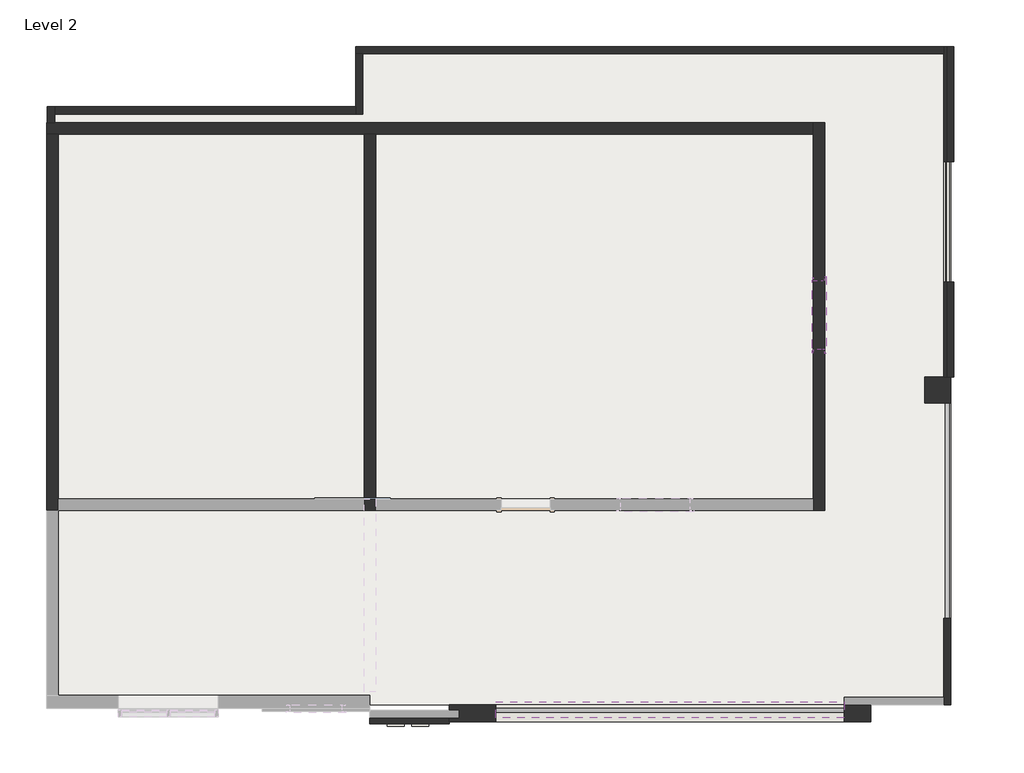
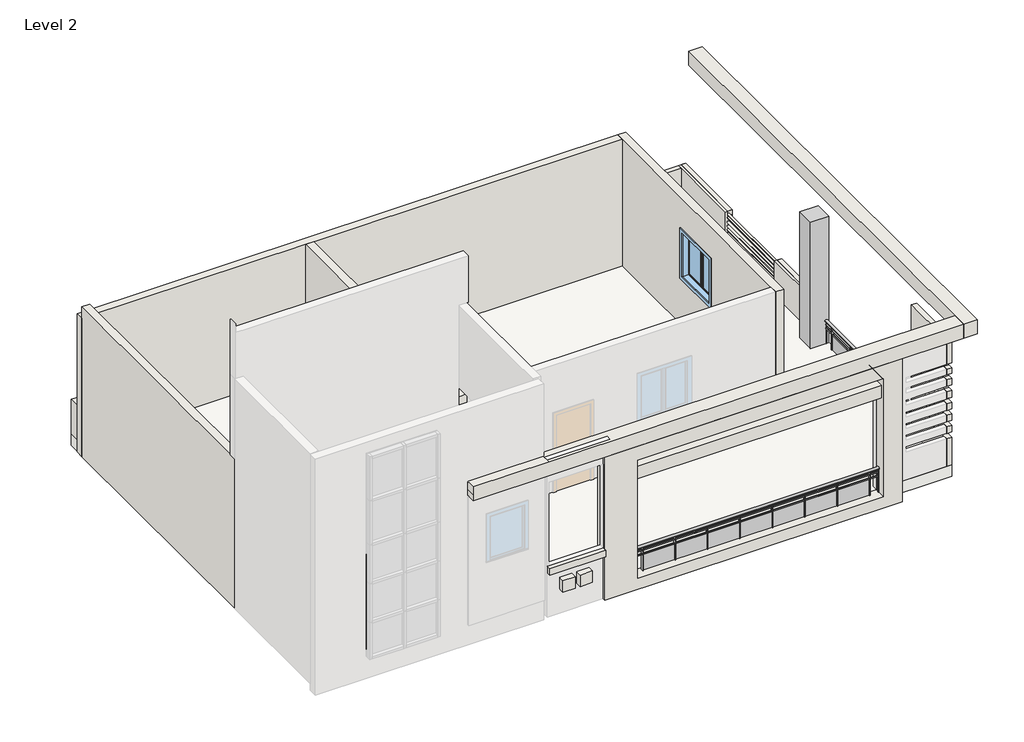
# One storey, part 2 of 2: 16 walls, 2 railings, 1 column, 1 roof, 1 window.
"""IFC4 building model written with IfcOpenShell, lengths in millimetres."""

from ifc_helpers import new_model, si_unit, point, frame, origin, place, context, project, spatial, polyline, ellipse_curve, trimmed, outline, extrude, faceted_brep, transform, mapped, element, save
from ifc_brep_helpers import plane_surface, extruded_surface, advanced_brep
from components import walls_1_walls_1_3d42d239, walls_4_walls_4_4fd3bbeb, walls_5_walls_5_3445876a, walls_6_walls_6_35ebc142, walls_7_walls_7_87e04c6a, walls_8_walls_8_d012f144, window_0862ab64

model = new_model("IFC4")

# Units and contexts
model_context = context("Model", 3, world=origin())
ifc_project = project(units=[si_unit("LENGTHUNIT", "METRE", prefix="MILLI")], contexts=[model_context])

# Site, building, storey
site = spatial("IfcSite", under=ifc_project)
building = spatial("IfcBuilding", under=site)
storey = spatial("IfcBuildingStorey", under=building, Name="Level 2", Elevation=3657.6)

# Column
placement = place(None, origin())
element("IfcColumn", 1, ObjectType="Rectangular Column : 18\" x 18\"", at=placement, inside=storey, context=model_context, shape_type="Brep", body=[
    faceted_brep([(2145.4271302, 2090.1740351, 7315.2), (1688.2271302, 2090.1740351, 7315.2), (1688.2271302, 1632.9740351, 7315.2), (2145.4271302, 1632.9740351, 7315.2), (2145.4271302, 2090.1740351, 3962.4), (2145.4271302, 1632.9740351, 3962.4), (1688.2271302, 1632.9740351, 3962.4), (1688.2271302, 2090.1740351, 3962.4), (2018.4271302, 2090.1740351, 3962.4), (2145.4271302, 2090.1740351, 4876.8)], [[[0, 1, 2, 3]], [[4, 5, 6, 7, 8]], [[1, 0, 9, 4, 8, 7]], [[2, 1, 7, 6]], [[3, 2, 6, 5]], [[0, 3, 5, 4, 9]]]),
])

# Railings
element("IfcRailing", 2, ObjectType="Glass Panel - Bottom Fill", at=placement, inside=storey, context=model_context, shape_type="SolidModel", body=[
    advanced_brep(
    [(-5897.2145744, -3764.5259649, 4605.5359375), (-5897.2145744, -3840.7259649, 4605.5359375), (258.2694807, -3764.5259649, 4605.5359375), (258.2694807, -3840.7259649, 4605.5359375)],
    [
        (0, 1, ellipse_curve(frame((-5897.2145744, -3802.6259649, 4605.5359375), z_axis=(-1.0, 0.0, 0.0), x_axis=(0.0, -1.0, 0.0)), 38.1, 28.575)),
        (1, 0, ellipse_curve(frame((-5897.2145744, -3802.6259649, 4605.5359375), z_axis=(-1.0, 0.0, 0.0), x_axis=(0.0, -1.0, 0.0)), 38.1, 28.575)),
        (2, 3, ellipse_curve(frame((258.2694807, -3802.6259649, 4605.5359375), z_axis=(1.0, 0.0, 0.0), x_axis=(0.0, -1.0, 0.0)), 38.1, 28.575)),
        (3, 2, ellipse_curve(frame((258.2694807, -3802.6259649, 4605.5359375), z_axis=(1.0, 0.0, 0.0), x_axis=(0.0, -1.0, 0.0)), 38.1, 28.575)),
        (0, 2),
        (3, 1),
    ],
    [
        plane_surface(frame((-5897.2145744, -3802.6259649, 4605.5359375), z_axis=(-1.0, 0.0, 0.0), x_axis=(0.0, 1.0, 0.0))),
        plane_surface(frame((258.2694807, -3802.6259649, 4605.5359375), z_axis=(1.0, 0.0, 0.0), x_axis=(0.0, 1.0, 0.0))),
        extruded_surface(trimmed(ellipse_curve(frame((258.2694807, -3802.6259649, 4605.5359375), z_axis=(-1.0, 0.0, 0.0), x_axis=(0.0, -1.0, 0.0)), 38.1, 28.575), [point((258.2694807, -3764.5259649, 4605.5359375))], [point((258.2694807, -3840.7259649, 4605.5359375))], True, "CARTESIAN"), (-6155.4840551, 0.0, 0.0), 6155.4840551),
        extruded_surface(trimmed(ellipse_curve(frame((258.2694807, -3802.6259649, 4605.5359375), z_axis=(-1.0, 0.0, 0.0), x_axis=(0.0, -1.0, 0.0)), 38.1, 28.575), [point((258.2694807, -3840.7259649, 4605.5359375))], [point((258.2694807, -3764.5259649, 4605.5359375))], True, "CARTESIAN"), (-6155.4840551, 0.0, 0.0), 6155.4840551),
    ],
    [
        (0, [[1, 2]]),
        (1, [[3, 4]]),
        (2, [[-1, 5, -4, 6]]),
        (3, [[-2, -6, -3, -5]]),
    ],
),
    extrude(outline(polyline([(-5897.2145744, -3815.3259649), (-5897.2145744, -3789.9259649), (258.2694807, -3789.9259649), (258.2694807, -3815.3259649), (-5897.2145744, -3815.3259649)])), frame((0.0, 0.0, 4491.2359375), z_axis=(0.0, 0.0, 1.0), x_axis=(1.0, 0.0, 0.0)), (0.0, 0.0, 1.0), 25.4),
    extrude(outline(polyline([(-5897.2145744, -3815.3259649), (-5897.2145744, -3789.9259649), (258.2694807, -3789.9259649), (258.2694807, -3815.3259649), (-5897.2145744, -3815.3259649)])), frame((0.0, 0.0, 4389.6359375), z_axis=(0.0, 0.0, 1.0), x_axis=(1.0, 0.0, 0.0)), (0.0, 0.0, 1.0), 25.4),
    extrude(outline(polyline([(18.9774532, -3828.0259649), (18.9774532, -3777.2259649), (31.6774532, -3777.2259649), (31.6774532, -3828.0259649), (18.9774532, -3828.0259649)])), frame((0.0, 0.0, 3691.1359375), z_axis=(0.0, 0.0, 1.0), x_axis=(1.0, 0.0, 0.0)), (0.0, 0.0, 1.0), 885.6788223),
    extrude(outline(polyline([(-787.4725468, -3796.0908079), (25.3274532, -3796.0908079), (25.3274532, -3802.4408079), (-787.4725468, -3802.4408079), (-787.4725468, -3796.0908079)])), frame((0.0, 0.0, 3792.7359375), z_axis=(0.0, 0.0, 1.0), x_axis=(1.0, 0.0, 0.0)), (0.0, 0.0, 1.0), 596.9),
    extrude(outline(polyline([(-793.8225468, -3828.0259649), (-793.8225468, -3777.2259649), (-781.1225468, -3777.2259649), (-781.1225468, -3828.0259649), (-793.8225468, -3828.0259649)])), frame((0.0, 0.0, 3691.1359375), z_axis=(0.0, 0.0, 1.0), x_axis=(1.0, 0.0, 0.0)), (0.0, 0.0, 1.0), 885.6788223),
    extrude(outline(polyline([(-1600.2725468, -3796.0908079), (-787.4725468, -3796.0908079), (-787.4725468, -3802.4408079), (-1600.2725468, -3802.4408079), (-1600.2725468, -3796.0908079)])), frame((0.0, 0.0, 3792.7359375), z_axis=(0.0, 0.0, 1.0), x_axis=(1.0, 0.0, 0.0)), (0.0, 0.0, 1.0), 596.9),
    extrude(outline(polyline([(-1606.6225468, -3828.0259649), (-1606.6225468, -3777.2259649), (-1593.9225468, -3777.2259649), (-1593.9225468, -3828.0259649), (-1606.6225468, -3828.0259649)])), frame((0.0, 0.0, 3691.1359375), z_axis=(0.0, 0.0, 1.0), x_axis=(1.0, 0.0, 0.0)), (0.0, 0.0, 1.0), 885.6788223),
    extrude(outline(polyline([(-2413.0725468, -3796.0908079), (-1600.2725468, -3796.0908079), (-1600.2725468, -3802.4408079), (-2413.0725468, -3802.4408079), (-2413.0725468, -3796.0908079)])), frame((0.0, 0.0, 3792.7359375), z_axis=(0.0, 0.0, 1.0), x_axis=(1.0, 0.0, 0.0)), (0.0, 0.0, 1.0), 596.9),
    extrude(outline(polyline([(-2419.4225468, -3828.0259649), (-2419.4225468, -3777.2259649), (-2406.7225468, -3777.2259649), (-2406.7225468, -3828.0259649), (-2419.4225468, -3828.0259649)])), frame((0.0, 0.0, 3691.1359375), z_axis=(0.0, 0.0, 1.0), x_axis=(1.0, 0.0, 0.0)), (0.0, 0.0, 1.0), 885.6788223),
    extrude(outline(polyline([(-3225.8725468, -3796.0908079), (-2413.0725468, -3796.0908079), (-2413.0725468, -3802.4408079), (-3225.8725468, -3802.4408079), (-3225.8725468, -3796.0908079)])), frame((0.0, 0.0, 3792.7359375), z_axis=(0.0, 0.0, 1.0), x_axis=(1.0, 0.0, 0.0)), (0.0, 0.0, 1.0), 596.9),
    extrude(outline(polyline([(-3232.2225468, -3828.0259649), (-3232.2225468, -3777.2259649), (-3219.5225468, -3777.2259649), (-3219.5225468, -3828.0259649), (-3232.2225468, -3828.0259649)])), frame((0.0, 0.0, 3691.1359375), z_axis=(0.0, 0.0, 1.0), x_axis=(1.0, 0.0, 0.0)), (0.0, 0.0, 1.0), 885.6788223),
    extrude(outline(polyline([(-4038.6725468, -3796.0908079), (-3225.8725468, -3796.0908079), (-3225.8725468, -3802.4408079), (-4038.6725468, -3802.4408079), (-4038.6725468, -3796.0908079)])), frame((0.0, 0.0, 3792.7359375), z_axis=(0.0, 0.0, 1.0), x_axis=(1.0, 0.0, 0.0)), (0.0, 0.0, 1.0), 596.9),
    extrude(outline(polyline([(-4045.0225468, -3828.0259649), (-4045.0225468, -3777.2259649), (-4032.3225468, -3777.2259649), (-4032.3225468, -3828.0259649), (-4045.0225468, -3828.0259649)])), frame((0.0, 0.0, 3691.1359375), z_axis=(0.0, 0.0, 1.0), x_axis=(1.0, 0.0, 0.0)), (0.0, 0.0, 1.0), 885.6788223),
    extrude(outline(polyline([(-4851.4725468, -3796.0908079), (-4038.6725468, -3796.0908079), (-4038.6725468, -3802.4408079), (-4851.4725468, -3802.4408079), (-4851.4725468, -3796.0908079)])), frame((0.0, 0.0, 3792.7359375), z_axis=(0.0, 0.0, 1.0), x_axis=(1.0, 0.0, 0.0)), (0.0, 0.0, 1.0), 596.9),
    extrude(outline(polyline([(-4857.8225468, -3828.0259649), (-4857.8225468, -3777.2259649), (-4845.1225468, -3777.2259649), (-4845.1225468, -3828.0259649), (-4857.8225468, -3828.0259649)])), frame((0.0, 0.0, 3691.1359375), z_axis=(0.0, 0.0, 1.0), x_axis=(1.0, 0.0, 0.0)), (0.0, 0.0, 1.0), 885.6788223),
    extrude(outline(polyline([(-5664.2725468, -3796.0908079), (-4851.4725468, -3796.0908079), (-4851.4725468, -3802.4408079), (-5664.2725468, -3802.4408079), (-5664.2725468, -3796.0908079)])), frame((0.0, 0.0, 3792.7359375), z_axis=(0.0, 0.0, 1.0), x_axis=(1.0, 0.0, 0.0)), (0.0, 0.0, 1.0), 596.9),
    extrude(outline(polyline([(-5670.6225468, -3828.0259649), (-5670.6225468, -3777.2259649), (-5657.9225468, -3777.2259649), (-5657.9225468, -3828.0259649), (-5670.6225468, -3828.0259649)])), frame((0.0, 0.0, 3691.1359375), z_axis=(0.0, 0.0, 1.0), x_axis=(1.0, 0.0, 0.0)), (0.0, 0.0, 1.0), 885.6788223),
    extrude(outline(polyline([(245.5694807, -3812.1509649), (245.5694807, -3793.1009649), (264.6194807, -3793.1009649), (264.6194807, -3812.1509649), (245.5694807, -3812.1509649)])), frame((0.0, 0.0, 3691.1359375), z_axis=(0.0, 0.0, 1.0), x_axis=(1.0, 0.0, 0.0)), (0.0, 0.0, 1.0), 885.6788223),
    extrude(outline(polyline([(-5903.5645744, -3812.1509649), (-5903.5645744, -3793.1009649), (-5884.5145744, -3793.1009649), (-5884.5145744, -3812.1509649), (-5903.5645744, -3812.1509649)])), frame((0.0, 0.0, 3691.1359375), z_axis=(0.0, 0.0, 1.0), x_axis=(1.0, 0.0, 0.0)), (0.0, 0.0, 1.0), 885.6788223),
])
element("IfcRailing", 3, ObjectType="Glass Panel - Bottom Fill", at=placement, inside=storey, context=model_context, shape_type="SolidModel", body=[
    advanced_brep(
    [(2043.8271302, -2177.0259649, 4572.0), (2120.0271302, -2177.0259649, 4572.0), (2043.8271302, 1632.9740351, 4572.0), (2120.0271302, 1632.9740351, 4572.0)],
    [
        (0, 1, ellipse_curve(frame((2081.9271302, -2177.0259649, 4572.0), z_axis=(0.0, -1.0, 0.0), x_axis=(1.0, 0.0, 0.0)), 38.1, 28.575)),
        (1, 0, ellipse_curve(frame((2081.9271302, -2177.0259649, 4572.0), z_axis=(0.0, -1.0, 0.0), x_axis=(1.0, 0.0, 0.0)), 38.1, 28.575)),
        (2, 3, ellipse_curve(frame((2081.9271302, 1632.9740351, 4572.0), z_axis=(0.0, 1.0, 0.0), x_axis=(1.0, 0.0, 0.0)), 38.1, 28.575)),
        (3, 2, ellipse_curve(frame((2081.9271302, 1632.9740351, 4572.0), z_axis=(0.0, 1.0, 0.0), x_axis=(1.0, 0.0, 0.0)), 38.1, 28.575)),
        (0, 2),
        (3, 1),
    ],
    [
        plane_surface(frame((2081.9271302, -2177.0259649, 4572.0), z_axis=(0.0, -1.0, 0.0), x_axis=(0.0, 0.0, 1.0))),
        plane_surface(frame((2081.9271302, 1632.9740351, 4572.0), z_axis=(0.0, 1.0, 0.0), x_axis=(0.0, 0.0, 1.0))),
        extruded_surface(trimmed(ellipse_curve(frame((2081.9271302, 1632.9740351, 4572.0), z_axis=(0.0, -1.0, 0.0), x_axis=(1.0, 0.0, 0.0)), 38.1, 28.575), [point((2043.8271302, 1632.9740351, 4572.0))], [point((2120.0271302, 1632.9740351, 4572.0))], True, "CARTESIAN"), (0.0, -3810.0, 0.0), 3810.0),
        extruded_surface(trimmed(ellipse_curve(frame((2081.9271302, 1632.9740351, 4572.0), z_axis=(0.0, -1.0, 0.0), x_axis=(1.0, 0.0, 0.0)), 38.1, 28.575), [point((2120.0271302, 1632.9740351, 4572.0))], [point((2043.8271302, 1632.9740351, 4572.0))], True, "CARTESIAN"), (0.0, -3810.0, 0.0), 3810.0),
    ],
    [
        (0, [[1, 2]]),
        (1, [[3, 4]]),
        (2, [[-1, 5, -4, 6]]),
        (3, [[-2, -6, -3, -5]]),
    ],
),
    extrude(outline(polyline([(2094.6271302, -2177.0259649), (2069.2271302, -2177.0259649), (2069.2271302, 1632.9740351), (2094.6271302, 1632.9740351), (2094.6271302, -2177.0259649)])), frame((0.0, 0.0, 4457.7), z_axis=(0.0, 0.0, 1.0), x_axis=(1.0, 0.0, 0.0)), (0.0, 0.0, 1.0), 25.4),
    extrude(outline(polyline([(2094.6271302, -2177.0259649), (2069.2271302, -2177.0259649), (2069.2271302, 1632.9740351), (2094.6271302, 1632.9740351), (2094.6271302, -2177.0259649)])), frame((0.0, 0.0, 4356.1), z_axis=(0.0, 0.0, 1.0), x_axis=(1.0, 0.0, 0.0)), (0.0, 0.0, 1.0), 25.4),
    extrude(outline(polyline([(2107.3271302, 1347.2240351), (2056.5271302, 1347.2240351), (2056.5271302, 1359.9240351), (2107.3271302, 1359.9240351), (2107.3271302, 1347.2240351)])), frame((0.0, 0.0, 3657.6), z_axis=(0.0, 0.0, 1.0), x_axis=(1.0, 0.0, 0.0)), (0.0, 0.0, 1.0), 885.6788223),
    extrude(outline(polyline([(2075.3919732, 540.7740351), (2075.3919732, 1353.5740351), (2081.7419732, 1353.5740351), (2081.7419732, 540.7740351), (2075.3919732, 540.7740351)])), frame((0.0, 0.0, 3759.2), z_axis=(0.0, 0.0, 1.0), x_axis=(1.0, 0.0, 0.0)), (0.0, 0.0, 1.0), 596.9),
    extrude(outline(polyline([(2107.3271302, 534.4240351), (2056.5271302, 534.4240351), (2056.5271302, 547.1240351), (2107.3271302, 547.1240351), (2107.3271302, 534.4240351)])), frame((0.0, 0.0, 3657.6), z_axis=(0.0, 0.0, 1.0), x_axis=(1.0, 0.0, 0.0)), (0.0, 0.0, 1.0), 885.6788223),
    extrude(outline(polyline([(2075.3919732, -272.0259649), (2075.3919732, 540.7740351), (2081.7419732, 540.7740351), (2081.7419732, -272.0259649), (2075.3919732, -272.0259649)])), frame((0.0, 0.0, 3759.2), z_axis=(0.0, 0.0, 1.0), x_axis=(1.0, 0.0, 0.0)), (0.0, 0.0, 1.0), 596.9),
    extrude(outline(polyline([(2107.3271302, -278.3759649), (2056.5271302, -278.3759649), (2056.5271302, -265.6759649), (2107.3271302, -265.6759649), (2107.3271302, -278.3759649)])), frame((0.0, 0.0, 3657.6), z_axis=(0.0, 0.0, 1.0), x_axis=(1.0, 0.0, 0.0)), (0.0, 0.0, 1.0), 885.6788223),
    extrude(outline(polyline([(2075.3919732, -1084.8259649), (2075.3919732, -272.0259649), (2081.7419732, -272.0259649), (2081.7419732, -1084.8259649), (2075.3919732, -1084.8259649)])), frame((0.0, 0.0, 3759.2), z_axis=(0.0, 0.0, 1.0), x_axis=(1.0, 0.0, 0.0)), (0.0, 0.0, 1.0), 596.9),
    extrude(outline(polyline([(2107.3271302, -1091.1759649), (2056.5271302, -1091.1759649), (2056.5271302, -1078.4759649), (2107.3271302, -1078.4759649), (2107.3271302, -1091.1759649)])), frame((0.0, 0.0, 3657.6), z_axis=(0.0, 0.0, 1.0), x_axis=(1.0, 0.0, 0.0)), (0.0, 0.0, 1.0), 885.6788223),
    extrude(outline(polyline([(2075.3919732, -1897.6259649), (2075.3919732, -1084.8259649), (2081.7419732, -1084.8259649), (2081.7419732, -1897.6259649), (2075.3919732, -1897.6259649)])), frame((0.0, 0.0, 3759.2), z_axis=(0.0, 0.0, 1.0), x_axis=(1.0, 0.0, 0.0)), (0.0, 0.0, 1.0), 596.9),
    extrude(outline(polyline([(2107.3271302, -1903.9759649), (2056.5271302, -1903.9759649), (2056.5271302, -1891.2759649), (2107.3271302, -1891.2759649), (2107.3271302, -1903.9759649)])), frame((0.0, 0.0, 3657.6), z_axis=(0.0, 0.0, 1.0), x_axis=(1.0, 0.0, 0.0)), (0.0, 0.0, 1.0), 885.6788223),
    extrude(outline(polyline([(2091.4521302, 1620.2740351), (2072.4021302, 1620.2740351), (2072.4021302, 1639.3240351), (2091.4521302, 1639.3240351), (2091.4521302, 1620.2740351)])), frame((0.0, 0.0, 3657.6), z_axis=(0.0, 0.0, 1.0), x_axis=(1.0, 0.0, 0.0)), (0.0, 0.0, 1.0), 885.6788223),
    extrude(outline(polyline([(2091.4521302, -2183.3759649), (2072.4021302, -2183.3759649), (2072.4021302, -2164.3259649), (2091.4521302, -2164.3259649), (2091.4521302, -2183.3759649)])), frame((0.0, 0.0, 3657.6), z_axis=(0.0, 0.0, 1.0), x_axis=(1.0, 0.0, 0.0)), (0.0, 0.0, 1.0), 885.6788223),
])

# Roof
element("IfcRoof", 4, ObjectType="Generic - 12\"", at=placement, inside=storey, context=model_context, shape_type="SweptSolid", body=[
    extrude(outline(polyline([(-13813.3305193, 6865.3740351), (-8370.1728698, 6865.3740351), (-8370.1728698, 7932.1740351), (2145.4271302, 7932.1740351), (2145.4271302, -3701.0259649), (-8249.5228698, -3701.0259649), (-8249.5228698, -3707.3759649), (-13813.3305193, -3707.3759649), (-13813.3305193, 6865.3740351)])), frame((0.0, 0.0, 3657.6), z_axis=(0.0, 0.0, 1.0), x_axis=(1.0, 0.0, 0.0)), (0.0, 0.0, 1.0), 304.8),
])

# Walls
element("IfcWall", 5, ObjectType="Generic - 5\"", at=placement, inside=storey, context=model_context, shape_type="Brep", body=[
    faceted_brep([(2145.4271302, -2177.0259649, 3962.4), (2145.4271302, -2177.0259649, 7315.2), (2145.4271302, -3574.0259649, 7315.2), (2145.4271302, -3701.0259649, 7315.2), (2145.4271302, -3701.0259649, 6665.1196283), (2145.4271302, -3574.0259649, 6665.1196283), (2145.4271302, -2570.7259649, 6665.1196283), (2145.4271302, -2570.7259649, 6538.1196283), (2145.4271302, -3574.0259649, 6538.1196283), (2145.4271302, -3701.0259649, 6538.1196283), (2145.4271302, -3701.0259649, 6385.7196283), (2145.4271302, -3637.5259649, 6385.7196283), (2145.4271302, -3637.5259649, 6380.7184058), (2145.4271302, -3574.0259649, 6380.7184058), (2145.4271302, -2570.7259649, 6380.7184058), (2145.4271302, -2570.7259649, 6253.7184058), (2145.4271302, -3574.0259649, 6253.7184058), (2145.4271302, -3701.0259649, 6253.7184058), (2145.4271302, -3701.0259649, 6080.9196283), (2145.4271302, -3637.5259649, 6080.9196283), (2145.4271302, -3637.5259649, 6075.9184058), (2145.4271302, -2570.7259649, 6075.9184058), (2145.4271302, -2570.7259649, 5942.5684058), (2145.4271302, -3574.0259649, 5942.5684058), (2145.4271302, -3701.0259649, 5942.5684058), (2145.4271302, -3701.0259649, 5753.1), (2145.4271302, -2570.7259649, 5753.1), (2145.4271302, -2570.7259649, 5621.3375), (2145.4271302, -3697.8509649, 5621.3375), (2145.4271302, -3697.8509649, 5442.5059058), (2145.4271302, -2570.7259649, 5442.5059058), (2145.4271302, -2570.7259649, 5313.9184058), (2145.4271302, -3701.0259649, 5313.9184058), (2145.4271302, -3701.0259649, 5141.1196283), (2145.4271302, -2570.7259649, 5141.1196283), (2145.4271302, -2570.7259649, 5010.9446283), (2145.4271302, -3701.0259649, 5010.9446283), (2145.4271302, -3701.0259649, 4832.9059058), (2145.4271302, -2570.7259649, 4832.9059058), (2145.4271302, -2570.7259649, 4691.6184058), (2145.4271302, -3701.0259649, 4691.6184058), (2145.4271302, -3701.0259649, 3962.4), (2018.4271302, -2177.0259649, 3962.4), (2018.4271302, -3574.0259649, 3962.4), (2018.4271302, -3701.0259649, 3962.4), (2018.4271302, -3701.0259649, 4691.6184058), (2018.4271302, -3574.0259649, 4691.6184058), (2018.4271302, -2570.7259649, 4691.6184058), (2018.4271302, -2570.7259649, 4832.9059058), (2018.4271302, -3701.0259649, 4832.9059058), (2018.4271302, -3701.0259649, 4836.3196283), (2018.4271302, -3701.0259649, 5009.1184058), (2018.4271302, -3701.0259649, 5010.9446283), (2018.4271302, -2570.7259649, 5010.9446283), (2018.4271302, -2570.7259649, 5141.1196283), (2018.4271302, -3574.0259649, 5141.1196283), (2018.4271302, -3701.0259649, 5141.1196283), (2018.4271302, -3701.0259649, 5313.9184058), (2018.4271302, -3574.0259649, 5313.9184058), (2018.4271302, -2570.7259649, 5313.9184058), (2018.4271302, -2570.7259649, 5442.5059058), (2018.4271302, -3697.8509649, 5442.5059058), (2018.4271302, -3697.8509649, 5621.3375), (2018.4271302, -2570.7259649, 5621.3375), (2018.4271302, -2570.7259649, 5753.1), (2018.4271302, -3574.0259649, 5753.1), (2018.4271302, -3701.0259649, 5753.1), (2018.4271302, -3701.0259649, 5936.2184058), (2018.4271302, -3701.0259649, 5942.5684058), (2018.4271302, -3574.0259649, 5942.5684058), (2018.4271302, -2570.7259649, 5942.5684058), (2018.4271302, -2570.7259649, 6075.9184058), (2018.4271302, -3637.5259649, 6075.9184058), (2018.4271302, -3637.5259649, 6080.9196283), (2018.4271302, -3701.0259649, 6080.9196283), (2018.4271302, -3701.0259649, 6253.7184058), (2018.4271302, -3574.0259649, 6253.7184058), (2018.4271302, -2570.7259649, 6253.7184058), (2018.4271302, -2570.7259649, 6380.7184058), (2018.4271302, -3574.0259649, 6380.7184058), (2018.4271302, -3637.5259649, 6380.7184058), (2018.4271302, -3637.5259649, 6385.7196283), (2018.4271302, -3701.0259649, 6385.7196283), (2018.4271302, -3701.0259649, 6533.1184058), (2018.4271302, -3701.0259649, 6538.1196283), (2018.4271302, -3574.0259649, 6538.1196283), (2018.4271302, -2570.7259649, 6538.1196283), (2018.4271302, -2570.7259649, 6665.1196283), (2018.4271302, -3574.0259649, 6665.1196283), (2018.4271302, -3701.0259649, 6665.1196283), (2018.4271302, -3701.0259649, 7315.2), (2018.4271302, -3574.0259649, 7315.2), (2018.4271302, -2177.0259649, 7315.2)], [[[0, 1, 2, 3, 4, 5, 6, 7, 8, 9, 10, 11, 12, 13, 14, 15, 16, 17, 18, 19, 20, 21, 22, 23, 24, 25, 26, 27, 28, 29, 30, 31, 32, 33, 34, 35, 36, 37, 38, 39, 40, 41]], [[42, 43, 44, 45, 46, 47, 48, 49, 50, 51, 52, 53, 54, 55, 56, 57, 58, 59, 60, 61, 62, 63, 64, 65, 66, 67, 68, 69, 70, 71, 72, 73, 74, 75, 76, 77, 78, 79, 80, 81, 82, 83, 84, 85, 86, 87, 88, 89, 90, 91, 92]], [[0, 41, 44, 43, 42]], [[1, 0, 42, 92]], [[2, 1, 92, 91]], [[3, 2, 91, 90]], [[5, 4, 89, 88]], [[6, 5, 88, 87]], [[7, 6, 87, 86]], [[8, 7, 86, 85]], [[9, 8, 85, 84]], [[13, 12, 80, 79]], [[14, 13, 79, 78]], [[15, 14, 78, 77]], [[16, 15, 77, 76]], [[17, 16, 76, 75]], [[21, 20, 72, 71]], [[22, 21, 71, 70]], [[23, 22, 70, 69]], [[24, 23, 69, 68]], [[25, 24, 68, 67, 66]], [[26, 25, 66, 65, 64]], [[27, 26, 64, 63]], [[28, 27, 63, 62]], [[29, 28, 62, 61]], [[30, 29, 61, 60]], [[31, 30, 60, 59]], [[32, 31, 59, 58, 57]], [[33, 32, 57, 56]], [[34, 33, 56, 55, 54]], [[35, 34, 54, 53]], [[36, 35, 53, 52]], [[37, 36, 52, 51, 50, 49]], [[38, 37, 49, 48]], [[39, 38, 48, 47]], [[40, 39, 47, 46, 45]], [[41, 40, 45, 44]], [[20, 19, 73, 72]], [[18, 74, 73, 19]], [[12, 11, 81, 80]], [[10, 82, 81, 11]], [[18, 17, 75, 74]], [[10, 9, 84, 83, 82]], [[4, 3, 90, 89]]]),
])
element("IfcWall", 6, ObjectType="Generic - 5\"", at=placement, inside=storey, context=model_context, shape_type="Brep", body=[
    faceted_brep([(2145.4271302, 2090.1740351, 3962.4), (2145.4271302, 7932.1740351, 3962.4), (2145.4271302, 7932.1740351, 4876.8), (2145.4271302, 5900.1740351, 4876.8), (2145.4271302, 5900.1740351, 4064.0), (2145.4271302, 3766.5740351, 4064.0), (2145.4271302, 3766.5740351, 4876.8), (2145.4271302, 2090.1740351, 4876.8), (2018.4271302, 2090.1740351, 3962.4), (2018.4271302, 2090.1740351, 4876.8), (2018.4271302, 3766.5740351, 4876.8), (2018.4271302, 3766.5740351, 4064.0), (2018.4271302, 5900.1740351, 4064.0), (2018.4271302, 5900.1740351, 4876.8), (2018.4271302, 7805.1740351, 4876.8), (2018.4271302, 7932.1740351, 4876.8), (2018.4271302, 7932.1740351, 3962.4), (2018.4271302, 7805.1740351, 3962.4)], [[[0, 1, 2, 3, 4, 5, 6, 7]], [[8, 9, 10, 11, 12, 13, 14, 15, 16, 17]], [[2, 1, 16, 15]], [[1, 0, 8, 17, 16]], [[0, 7, 9, 8]], [[3, 2, 15, 14, 13]], [[4, 3, 13, 12]], [[5, 4, 12, 11]], [[6, 5, 11, 10]], [[7, 6, 10, 9]]]),
])
element("IfcWall", 7, ObjectType="Generic - 5\"", at=placement, inside=storey, context=model_context, shape_type="Brep", body=[
    faceted_brep([(2018.4271302, 7932.1740351, 3962.4), (-8370.1728698, 7932.1740351, 3962.4), (-8370.1728698, 7932.1740351, 4876.8), (2018.4271302, 7932.1740351, 4876.8), (2018.4271302, 7805.1740351, 3962.4), (2018.4271302, 7805.1740351, 4876.8), (-8243.1728698, 7805.1740351, 4876.8), (-8370.1728698, 7805.1740351, 4876.8), (-8370.1728698, 7805.1740351, 3962.4), (-8243.1728698, 7805.1740351, 3962.4)], [[[0, 1, 2, 3]], [[4, 5, 6, 7, 8, 9]], [[1, 0, 4, 9, 8]], [[3, 2, 7, 6, 5]], [[0, 3, 5, 4]], [[2, 1, 8, 7]]]),
])
element("IfcWall", 8, ObjectType="Generic - 5\"", at=placement, inside=storey, context=model_context, shape_type="Brep", body=[
    faceted_brep([(-8370.1728698, 7805.1740351, 3962.4), (-8370.1728698, 6865.3740351, 3962.4), (-8370.1728698, 6738.3740351, 3962.4), (-8370.1728698, 6738.3740351, 4876.8), (-8370.1728698, 6865.3740351, 4876.8), (-8370.1728698, 7805.1740351, 4876.8), (-8243.1728698, 7805.1740351, 3962.4), (-8243.1728698, 7805.1740351, 4876.8), (-8243.1728698, 6738.3740351, 4876.8), (-8243.1728698, 6738.3740351, 3962.4)], [[[0, 1, 2, 3, 4, 5]], [[6, 7, 8, 9]], [[2, 1, 0, 6, 9]], [[5, 4, 3, 8, 7]], [[0, 5, 7, 6]], [[3, 2, 9, 8]]]),
])
element("IfcWall", 9, ObjectType="Generic - 5\"", at=placement, inside=storey, context=model_context, shape_type="SweptSolid", body=[
    extrude(outline(polyline([(-13686.3305193, 6865.3740351), (-8370.1728698, 6865.3740351), (-8370.1728698, 6738.3740351), (-13686.3305193, 6738.3740351), (-13686.3305193, 6865.3740351)])), frame((0.0, 0.0, 3962.4), z_axis=(0.0, 0.0, 1.0), x_axis=(1.0, 0.0, 0.0)), (0.0, 0.0, 1.0), 914.4),
])
element("IfcWall", 10, ObjectType="Generic - 5\"", at=placement, inside=storey, context=model_context, shape_type="Brep", body=[
    faceted_brep([(-13813.3305193, 6865.3740351, 3962.4), (-13813.3305193, 6585.9740351, 3962.4), (-13813.3305193, 6585.9740351, 4876.8), (-13813.3305193, 6865.3740351, 4876.8), (-13686.3305193, 6865.3740351, 3962.4), (-13686.3305193, 6865.3740351, 4876.8), (-13686.3305193, 6738.3740351, 4876.8), (-13686.3305193, 6585.9740351, 4876.8), (-13686.3305193, 6585.9740351, 3962.4), (-13686.3305193, 6738.3740351, 3962.4)], [[[0, 1, 2, 3]], [[4, 5, 6, 7, 8, 9]], [[1, 0, 4, 9, 8]], [[3, 2, 7, 6, 5]], [[0, 3, 5, 4]], [[2, 1, 8, 7]]]),
])
element("IfcWall", 11, ObjectType="Generic - 8\"", at=placement, inside=storey, context=model_context, shape_type="Brep", body=[
    faceted_brep([(-284.932483, 6585.9740351, 3657.6), (-284.932483, 6382.7740351, 3657.6), (-284.932483, -68.8259649, 3657.6), (-284.932483, -272.0259649, 3657.6), (-284.932483, -272.0259649, 7315.2), (-284.932483, -68.8259649, 7315.2), (-284.932483, 6382.7740351, 7315.2), (-284.932483, 6585.9740351, 7315.2), (-284.932483, 2572.7740351, 6462.0860139), (-284.932483, 2572.7740351, 5242.8860139), (-284.932483, 3791.9740351, 5242.8860139), (-284.932483, 3791.9740351, 6462.0860139), (-81.732483, 6585.9740351, 3657.6), (-81.732483, 6585.9740351, 7315.2), (-81.732483, -272.0259649, 7315.2), (-81.732483, -272.0259649, 3657.6), (-81.732483, 2572.7740351, 6462.0860139), (-81.732483, 3791.9740351, 6462.0860139), (-81.732483, 3791.9740351, 5242.8860139), (-81.732483, 2572.7740351, 5242.8860139)], [[[0, 1, 2, 3, 4, 5, 6, 7], [8, 9, 10, 11]], [[12, 13, 14, 15], [16, 17, 18, 19]], [[3, 2, 1, 0, 12, 15]], [[7, 6, 5, 4, 14, 13]], [[0, 7, 13, 12]], [[4, 3, 15, 14]], [[9, 8, 16, 19]], [[10, 9, 19, 18]], [[11, 10, 18, 17]], [[8, 11, 17, 16]]]),
])
element("IfcWall", 12, ObjectType="Generic - 8\"", at=placement, inside=storey, context=model_context, shape_type="Brep", body=[
    faceted_brep([(-8217.7728698, 6382.7740351, 3657.6), (-8217.7728698, -68.8259649, 3657.6), (-8217.7728698, -272.0259649, 3657.6), (-8217.7728698, -272.0259649, 4889.3737543), (-8217.7728698, -68.8259649, 4889.3737543), (-8217.7728698, -68.8259649, 6108.5737543), (-8217.7728698, -272.0259649, 6108.5737543), (-8217.7728698, -272.0259649, 7315.2), (-8217.7728698, 6382.7740351, 7315.2), (-8014.5728698, -272.0259649, 3657.6), (-8014.5728698, -68.8259649, 3657.6), (-8014.5728698, 6382.7740351, 3657.6), (-8014.5728698, 6382.7740351, 7315.2), (-8014.5728698, -68.8259649, 7315.2), (-8014.5728698, -272.0259649, 7315.2), (-8014.5728698, -272.0259649, 6108.5737543), (-8014.5728698, -68.8259649, 6108.5737543), (-8014.5728698, -68.8259649, 4889.3737543), (-8014.5728698, -272.0259649, 4889.3737543)], [[[0, 1, 2, 3, 4, 5, 6, 7, 8]], [[9, 10, 11, 12, 13, 14, 15, 16, 17, 18]], [[2, 1, 0, 11, 10, 9]], [[8, 7, 14, 13, 12]], [[0, 8, 12, 11]], [[2, 9, 18, 3]], [[14, 7, 6, 15]], [[4, 17, 16, 5]], [[17, 4, 3, 18]], [[5, 16, 15, 6]]]),
])
element("IfcWall", 13, ObjectType="Generic - 8\"", at=placement, inside=storey, context=model_context, shape_type="Brep", body=[
    faceted_brep([(-13824.8228698, 6382.7740351, 7315.2), (-13824.8228698, 6382.7740351, 3657.6), (-13621.6228698, 6382.7740351, 3657.6), (-8217.7728698, 6382.7740351, 3657.6), (-8014.5728698, 6382.7740351, 3657.6), (-284.932483, 6382.7740351, 3657.6), (-284.932483, 6382.7740351, 7315.2), (-8014.5728698, 6382.7740351, 7315.2), (-8217.7728698, 6382.7740351, 7315.2), (-13824.8228698, 6585.9740351, 3657.6), (-13824.8228698, 6585.9740351, 7315.2), (-284.932483, 6585.9740351, 7315.2), (-284.932483, 6585.9740351, 3657.6)], [[[0, 1, 2, 3, 4, 5, 6, 7, 8]], [[9, 10, 11, 12]], [[5, 4, 3, 2, 1, 9, 12]], [[0, 8, 7, 6, 11, 10]], [[6, 5, 12, 11]], [[0, 10, 9, 1]]]),
])
element("IfcWall", 14, ObjectType="Generic - 8\"", at=placement, inside=storey, context=model_context, shape_type="Brep", body=[
    faceted_brep([(-13824.8228698, 6382.7740351, 7620.0), (-13824.8228698, 6382.7740351, 7315.2), (-13824.8228698, 6382.7740351, 3657.6), (-13824.8228698, -272.0259649, 3657.6), (-13824.8228698, -272.0259649, 7620.0), (-13621.6228698, 6382.7740351, 3657.6), (-13621.6228698, 6382.7740351, 7620.0), (-13621.6228698, -68.8259649, 7620.0), (-13621.6228698, -272.0259649, 7620.0), (-13621.6228698, -272.0259649, 3657.6), (-13621.6228698, -68.8259649, 3657.6), (-13626.0055193, -272.0259649, 3657.6)], [[[0, 1, 2, 3, 4]], [[5, 6, 7, 8, 9, 10]], [[4, 3, 11, 9, 8]], [[3, 2, 5, 10, 9, 11]], [[0, 4, 8, 7, 6]], [[0, 6, 5, 2, 1]]]),
])
walls_1_walls_1_shape = walls_1_walls_1_3d42d239(model_context)
element("IfcWall", 15, ObjectType="Walls 1 : Walls 1", at=placement, inside=storey, context=model_context, shape_type="MappedRepresentation", body=[
    mapped(walls_1_walls_1_shape, transform((0.0, 0.0, 0.0), x_axis=(1.0, 0.0, 0.0), y_axis=(0.0, 1.0, 0.0), z_axis=(0.0, 0.0, 1.0))),
])
walls_4_walls_4_shape = walls_4_walls_4_4fd3bbeb(model_context)
element("IfcWall", 16, ObjectType="Walls 4 : Walls 4", at=placement, inside=storey, context=model_context, shape_type="MappedRepresentation", body=[
    mapped(walls_4_walls_4_shape, transform((0.0, 0.0, 0.0), x_axis=(1.0, 0.0, 0.0), y_axis=(0.0, 1.0, 0.0), z_axis=(0.0, 0.0, 1.0))),
])
walls_5_walls_5_shape = walls_5_walls_5_3445876a(model_context)
element("IfcWall", 17, ObjectType="Walls 5 : Walls 5", at=placement, inside=storey, context=model_context, shape_type="MappedRepresentation", body=[
    mapped(walls_5_walls_5_shape, transform((0.0, 0.0, 0.0), x_axis=(1.0, 0.0, 0.0), y_axis=(0.0, 1.0, 0.0), z_axis=(0.0, 0.0, 1.0))),
])
walls_6_walls_6_shape = walls_6_walls_6_35ebc142(model_context)
element("IfcWall", 18, ObjectType="Walls 6 : Walls 6", at=placement, inside=storey, context=model_context, shape_type="MappedRepresentation", body=[
    mapped(walls_6_walls_6_shape, transform((0.0, 0.0, 0.0), x_axis=(1.0, 0.0, 0.0), y_axis=(0.0, 1.0, 0.0), z_axis=(0.0, 0.0, 1.0))),
])
walls_7_walls_7_shape = walls_7_walls_7_87e04c6a(model_context)
element("IfcWall", 19, ObjectType="Walls 7 : Walls 7", at=placement, inside=storey, context=model_context, shape_type="MappedRepresentation", body=[
    mapped(walls_7_walls_7_shape, transform((0.0, 0.0, 0.0), x_axis=(1.0, 0.0, 0.0), y_axis=(0.0, 1.0, 0.0), z_axis=(0.0, 0.0, 1.0))),
])
walls_8_walls_8_shape = walls_8_walls_8_d012f144(model_context)
element("IfcWall", 20, ObjectType="Walls 8 : Walls 8", at=placement, inside=storey, context=model_context, shape_type="MappedRepresentation", body=[
    mapped(walls_8_walls_8_shape, transform((0.0, 0.0, 0.0), x_axis=(1.0, 0.0, 0.0), y_axis=(0.0, 1.0, 0.0), z_axis=(0.0, 0.0, 1.0))),
])

# Window
window_shape = window_0862ab64(model_context)
element("IfcWindow", 21, ObjectType="Casement Dbl with Trim : 48\" x 48\"", at=placement, inside=storey, context=model_context, shape_type="MappedRepresentation", body=[
    mapped(window_shape, transform((-202.382483, 3182.3740351, 4328.4860139), x_axis=(0.0, -1.0, 0.0), y_axis=(1.0, 0.0, 0.0), z_axis=(0.0, 0.0, 1.0))),
])

save(model, "model.ifc")

# Revit data of these elements
# Type "Rectangular Column : 18\" x 18\""
#   Assembly Code = "B1010200"
#   Depth = 1' - 6"
#   Offset Base = 0' - 0"
#   Offset Top = 0' - 0"
#   Width = 1' - 6"
#   Material = none
# Type "Glass Panel - Bottom Fill"
#   Assembly Code = "C2010400"
#   built-in parameter 1008612 = 0.0416667 (stored number, unit not read)
#   built-in parameter 1008611 = 0.0416667 (stored number, unit not read)
#   built-in parameter 1008609 = 0.333333 (stored number, unit not read)
#   built-in parameter 1008604 = 0.166667 (stored number, unit not read)
#   built-in parameter 1008603 = 0.166667 (stored number, unit not read)
#   Railing Height = 3' - 0"
#   built-in parameter 1008630 = 2
#   built-in parameter 1008610 = 2
#   built-in parameter 1008618 = Baluster - Square : 3/4"
# Type "Generic - 12\""
#   Assembly Code = "B1020"
#   Layers, outside or top first: 1' - 0" no material (function 1)
# Type "Generic - 5\""
#   Assembly Code = "B2010"
#   Layers, outside or top first: 0' - 5" no material (function 1)
# Type "Generic - 8\""
#   Assembly Code = "B2010"
#   Layers, outside or top first: 0' - 8" no material (function 1)
# Type "Casement Dbl with Trim : 48\" x 48\""
#   Type Mark = "19"
#   Construction Type Id = "GSP4R"
#   Assembly Code = "B2020100"
#   Analytic Construction = "1/8 in Pilkington single glazing"
#   Visual Light Transmittance = 0.9
#   Solar Heat Gain Coefficient = 0.78
#   Heat Transfer Coefficient (U) = 0.6496 BTU/(h·ft²·°F)
#   Height = 4' - 0"
#   Default Sill Height = 3' - 0"
#   Trim Projection - Ext. = 0' - 0 1/2"
#   Trim Projection - Int. = 0' - 0 3/4"
#   Trim Width - Exterior = 0' - 3 1/2"
#   Trim Width - Interior = 0' - 3 1/2"
#   Width = 4' - 0"
#   Window Inset = 0' - 0 3/4"
#   Define Thermal Properties by = 1
#   Glass Pane Material = Glass
#   Sash Material = Sash
#   Trim Exterior Material = Trim
#   Trim Interior Material = Trim
#   Wall Closure = (empty or 0)
# Element 1 (IfcColumn, "Rectangular Column : 18\" x 18\"")
#   Phase Created = New Construction
#   Materials on its faces: "Default Wall"
# Element 2 (IfcRailing, "Glass Panel - Bottom Fill")
#   built-in parameter 1008621 = 0.110026 (stored number, unit not read)
#   Phase Created = New Construction
#   Materials on its faces: "Glass"
# Element 3 (IfcRailing, "Glass Panel - Bottom Fill")
#   Phase Created = New Construction
#   Materials on its faces: "Glass"
# Element 4 (IfcRoof, "Generic - 12\"")
#   built-in parameter 1001705 = 13 (stored number, unit not read)
#   built-in parameter 1001710 = 33615
#   Phase Created = New Construction
#   Materials on its faces: "Default Roof"
# Element 5 (IfcWall, "Generic - 5\"")
#   built-in parameter 1001111 = 1' - 0"
#   Top Offset = 0' - 0"
#   Base Offset = 1' - 0"
#   wall height = 11' - 0"
#   Phase Created = New Construction
#   Base Constraint = Level 2
#   Top Constraint = Level 3
#   Materials on its faces: "Default Wall"
# Elements 6, 7, 8, 9, 10 (IfcWall, "Generic - 5\"")
#   built-in parameter 1001111 = 1' - 0"
#   Top Offset = -8' - 0"
#   Base Offset = 1' - 0"
#   wall height = 3' - 0"
#   Phase Created = New Construction
#   Base Constraint = Level 2
#   Top Constraint = Level 3
#   Materials on its faces: "Default Wall"
# Elements 11, 12, 13 (IfcWall, "Generic - 8\"")
#   Top Offset = 0' - 0"
#   Base Offset = 0' - 0"
#   Unconnected Height = 12' - 0"
#   wall height = 12' - 0"
#   Phase Created = New Construction
#   Base Constraint = Level 2
#   Materials on its faces: "Default Wall"
# Element 14 (IfcWall, "Generic - 8\"")
#   Top Offset = 0' - 0"
#   Base Offset = 0' - 0"
#   Unconnected Height = 13' - 0"
#   wall height = 13' - 0"
#   Phase Created = New Construction
#   Base Constraint = Level 2
#   Materials on its faces: "Default Wall"
# Element 15 (IfcWall, "Walls 1 : Walls 1")
#   Phase Created = New Construction
#   Materials on its faces: "Default Wall"
# Element 16 (IfcWall, "Walls 4 : Walls 4")
#   Phase Created = New Construction
#   Materials on its faces: "Default Wall"
# Element 17 (IfcWall, "Walls 5 : Walls 5")
#   Phase Created = New Construction
#   Materials on its faces: "Default Wall"
# Element 18 (IfcWall, "Walls 6 : Walls 6")
#   Phase Created = New Construction
#   Materials on its faces: "Default Wall"
# Element 19 (IfcWall, "Walls 7 : Walls 7")
#   Phase Created = New Construction
#   Materials on its faces: "Default Wall"
# Element 20 (IfcWall, "Walls 8 : Walls 8")
#   Phase Created = New Construction
#   Materials on its faces: "Default Wall"
# Element 21 (IfcWindow, "Casement Dbl with Trim : 48\" x 48\"")
#   Mark = "7"
#   Phase Created = New Construction
#   Materials on its faces: "Sash", "Trim", "Glass"
# Materials
#   "Glass": class "Glass", colour RGB 0 128 192, transparency 0.75, Description = "Soda Lime Glass", Cost = 0
#   "Sash": class "Wood", colour RGB 224 178 126, transparency 0
#   "Trim": class "Wood", colour RGB 224 178 126, transparency 0
#   "Default Wall": colour RGB 128 128 128, transparency 0
#   "Default Roof": colour RGB 88 101 114, transparency 0
